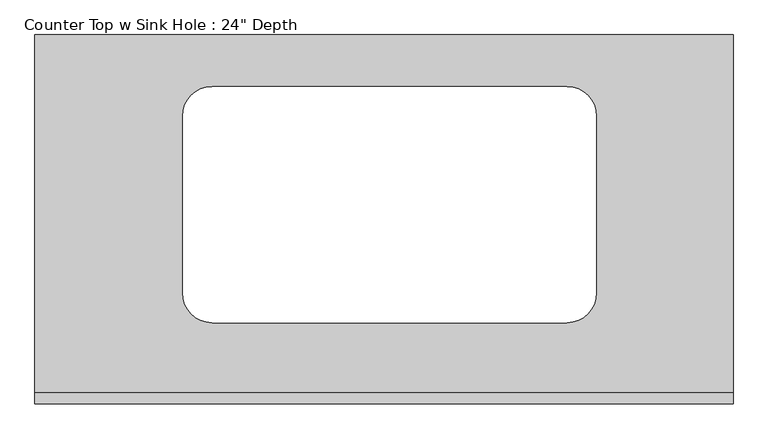
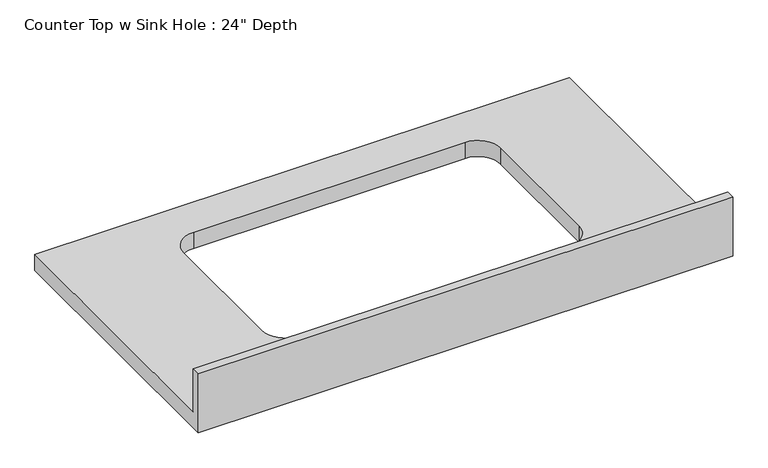
"""IFC4 building model written with IfcOpenShell, lengths in millimetres: furniture geometry."""

from ifc_helpers import new_model, si_unit, frame, origin, place, context, project, spatial, polyline, circle_curve, source, transform, mapped, element, save
from ifc_brep_helpers import plane_surface, revolved_surface, advanced_brep


def furniture_49e6720b(model_context):
    return source(origin(), model_context, "Body", "AdvancedBrep", [
        advanced_brep(
        [(-1200.4622951, 635.0, 914.4), (-1200.4622951, 19.05, 914.4), (-0.130724, 19.05, 914.4), (-0.130724, 635.0, 914.4), (-895.6622951, 139.7, 914.4), (-946.4622951, 190.5, 914.4), (-946.4622951, 495.3, 914.4), (-895.6622951, 546.1, 914.4), (-286.0622951, 546.1, 914.4), (-235.2622951, 495.3, 914.4), (-235.2622951, 190.5, 914.4), (-286.0622951, 139.7, 914.4), (-0.130724, 0.0, 876.3), (-1200.4622951, 0.0, 876.3), (-1200.4622951, 635.0, 876.3), (-0.130724, 635.0, 876.3), (-286.0622951, 139.7, 876.3), (-235.2622951, 190.5, 876.3), (-235.2622951, 495.3, 876.3), (-286.0622951, 546.1, 876.3), (-895.6622951, 546.1, 876.3), (-946.4622951, 495.3, 876.3), (-946.4622951, 190.5, 876.3), (-895.6622951, 139.7, 876.3), (-0.130724, 0.0, 1016.0), (-1200.4622951, 0.0, 1016.0), (-1200.4622951, 19.05, 1016.0), (-0.130724, 19.05, 1016.0)],
        [
            (0, 1),
            (1, 2),
            (2, 3),
            (3, 0),
            (4, 5, circle_curve(frame((-895.6622951, 190.5, 914.4), z_axis=(0.0, 0.0, -1.0), x_axis=(1.0, 0.0, 0.0)), 50.8)),
            (5, 6),
            (6, 7, circle_curve(frame((-895.6622951, 495.3, 914.4), z_axis=(0.0, 0.0, -1.0), x_axis=(1.0, 0.0, 0.0)), 50.8)),
            (7, 8),
            (8, 9, circle_curve(frame((-286.0622951, 495.3, 914.4), z_axis=(0.0, 0.0, -1.0), x_axis=(1.0, 0.0, 0.0)), 50.8)),
            (9, 10),
            (10, 11, circle_curve(frame((-286.0622951, 190.5, 914.4), z_axis=(0.0, 0.0, -1.0), x_axis=(1.0, 0.0, 0.0)), 50.8)),
            (11, 4),
            (12, 13),
            (13, 14),
            (14, 15),
            (15, 12),
            (16, 17, circle_curve(frame((-286.0622951, 190.5, 876.3), z_axis=(0.0, 0.0, 1.0), x_axis=(1.0, 0.0, 0.0)), 50.8)),
            (17, 18),
            (18, 19, circle_curve(frame((-286.0622951, 495.3, 876.3), z_axis=(0.0, 0.0, 1.0), x_axis=(1.0, 0.0, 0.0)), 50.8)),
            (19, 20),
            (20, 21, circle_curve(frame((-895.6622951, 495.3, 876.3), z_axis=(0.0, 0.0, 1.0), x_axis=(1.0, 0.0, 0.0)), 50.8)),
            (21, 22),
            (22, 23, circle_curve(frame((-895.6622951, 190.5, 876.3), z_axis=(0.0, 0.0, 1.0), x_axis=(1.0, 0.0, 0.0)), 50.8)),
            (23, 16),
            (12, 24),
            (24, 25),
            (25, 13),
            (25, 26),
            (26, 1),
            (0, 14),
            (3, 15),
            (2, 27),
            (27, 24),
            (27, 26),
            (11, 16),
            (23, 4),
            (22, 5),
            (21, 6),
            (20, 7),
            (19, 8),
            (18, 9),
            (17, 10),
        ],
        [
            plane_surface(frame((-1200.4622951, 0.0, 914.4), z_axis=(0.0, 0.0, 1.0), x_axis=(-1.0, 0.0, 0.0))),
            plane_surface(frame((-1200.4622951, 0.0, 876.3), z_axis=(0.0, 0.0, -1.0), x_axis=(1.0, 0.0, 0.0))),
            plane_surface(frame((-0.130724, 0.0, 914.4), z_axis=(0.0, -1.0, 0.0), x_axis=(0.0, 0.0, -1.0))),
            plane_surface(frame((-1200.4622951, 0.0, 914.4), z_axis=(-1.0, 0.0, 0.0), x_axis=(0.0, 0.0, -1.0))),
            plane_surface(frame((-1200.4622951, 635.0, 914.4), z_axis=(0.0, 1.0, 0.0), x_axis=(0.0, 0.0, -1.0))),
            plane_surface(frame((-0.130724, 635.0, 914.4), z_axis=(1.0, 0.0, 0.0), x_axis=(0.0, 0.0, -1.0))),
            plane_surface(frame((-1200.4622951, 0.0, 1016.0), z_axis=(0.0, 0.0, 1.0), x_axis=(0.0, 1.0, 0.0))),
            plane_surface(frame((-1200.4622951, 19.05, 1016.0), z_axis=(0.0, 1.0, 0.0), x_axis=(0.0, 0.0, -1.0))),
            plane_surface(frame((-286.0622951, 139.7, 914.4), z_axis=(0.0, 1.0, 0.0), x_axis=(0.0, 0.0, -1.0))),
            revolved_surface(polyline([(-844.8622951000001, 190.5, 914.4), (-844.8622951000001, 190.5, 876.3)]), (-895.6622951, 190.5, 876.3), (0.0, 0.0, 1.0)),
            plane_surface(frame((-946.4622951, 190.5, 914.4), z_axis=(1.0, 0.0, 0.0), x_axis=(0.0, 0.0, -1.0))),
            revolved_surface(polyline([(-844.8622951000001, 495.3, 914.4), (-844.8622951000001, 495.3, 876.3)]), (-895.6622951, 495.3, 876.3), (0.0, 0.0, 1.0)),
            plane_surface(frame((-895.6622951, 546.1, 914.4), z_axis=(0.0, -1.0, 0.0), x_axis=(0.0, 0.0, -1.0))),
            revolved_surface(polyline([(-235.26229509999996, 495.3, 914.4), (-235.26229509999996, 495.3, 876.3)]), (-286.0622951, 495.3, 876.3), (0.0, 0.0, 1.0)),
            plane_surface(frame((-235.2622951, 495.3, 914.4), z_axis=(-1.0, 0.0, 0.0), x_axis=(0.0, 0.0, -1.0))),
            revolved_surface(polyline([(-235.26229509999996, 190.5, 914.4), (-235.26229509999996, 190.5, 876.3)]), (-286.0622951, 190.5, 876.3), (0.0, 0.0, 1.0)),
        ],
        [
            (0, [[1, 2, 3, 4], [5, 6, 7, 8, 9, 10, 11, 12]]),
            (1, [[13, 14, 15, 16], [17, 18, 19, 20, 21, 22, 23, 24]]),
            (2, [[25, 26, 27, -13]]),
            (3, [[-27, 28, 29, -1, 30, -14]]),
            (4, [[31, -15, -30, -4]]),
            (5, [[-31, -3, 32, 33, -25, -16]]),
            (6, [[-26, -33, 34, -28]]),
            (7, [[-32, -2, -29, -34]]),
            (8, [[-12, 35, -24, 36]]),
            (9, [[-23, 37, -5, -36]]),
            (10, [[-22, 38, -6, -37]]),
            (11, [[-21, 39, -7, -38]]),
            (12, [[-20, 40, -8, -39]]),
            (13, [[-19, 41, -9, -40]]),
            (14, [[-18, 42, -10, -41]]),
            (15, [[-11, -42, -17, -35]]),
        ],
    ),
    ])


if __name__ == "__main__":
    model = new_model("IFC4")
    model_context = context("Model", 3, world=origin())
    ifc_project = project(units=[si_unit("LENGTHUNIT", "METRE", prefix="MILLI")], contexts=[model_context])
    site = spatial("IfcSite", under=ifc_project)
    building = spatial("IfcBuilding", under=site)
    placement = place(None, origin())
    furniture_shape = furniture_49e6720b(model_context)
    element("IfcFurniture", 1, ObjectType="Counter Top w Sink Hole : 24\" Depth", at=placement, inside=building, context=model_context, shape_type="MappedRepresentation", body=[
        mapped(furniture_shape, transform((0.0, 0.0, 0.0), x_axis=(1.0, 0.0, 0.0), y_axis=(0.0, 1.0, 0.0), z_axis=(0.0, 0.0, 1.0))),
    ])
    save(model, "model.ifc")

# Revit data of these elements
# Type "Counter Top w Sink Hole : 24\" Depth"
#   Assembly Code = "C1030400"
#   Counter Thickness = 0' - 1 1/2"
#   Depth = 2' - 1"
#   Height = 3' - 0"
#   Length [instance default] = 8' - 0"
#   Sink Location [instance default] = 2' - 0"
#   Sink Location To Wall [instance default] = 0' - 6"
#   Sink Opening Depth [instance default] = 1' - 3"
#   Sink Opening Width [instance default] = 2' - 3"
#   Counter Top Material = none
#   Default Elevation = 0
# Element 1 (IfcFurniture, "Counter Top w Sink Hole : 24\" Depth")
#   Length = 3' - 11.25715"
#   Materials on its faces: "Counter Top"
# Materials
#   "Counter Top": class "Wood", colour RGB 226 177 128, transparency 0
